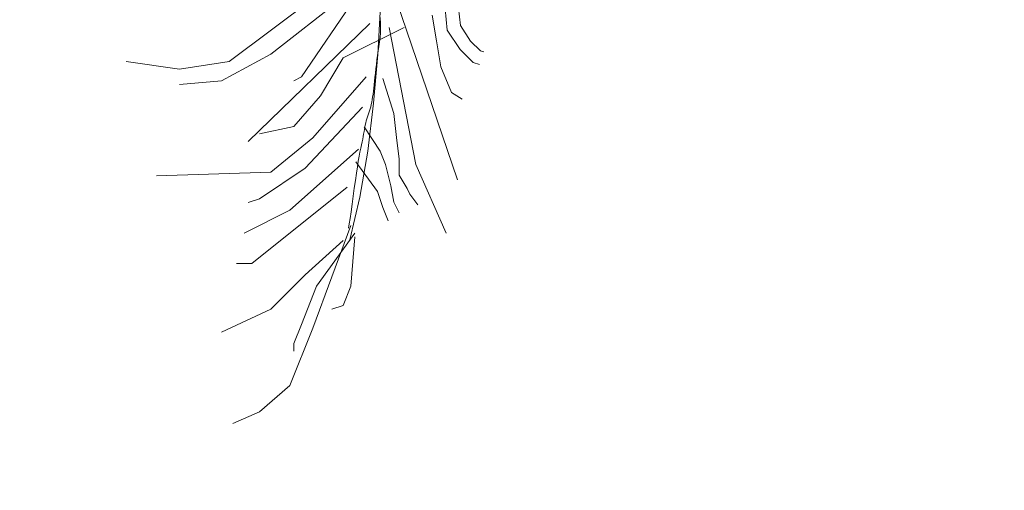
# Model space of a CAD drawing. Units: millimetres. Extents: x 595116 to 630915, y 909473 to 920225.
# Tile 83 of 134: x 629720.161 to 629727.558, y 919266.512 to 919270.048. Entities that reach past the tile are written whole.
import ezdxf

# ---------------------------------------------------------------- set-up
doc = ezdxf.new("R2010")
doc.units = ezdxf.units.MM
doc.layers.add('Dimension', color=3, linetype='Continuous', lineweight=18)
doc.layers.add('L-PLNT', color=85, linetype='Continuous', lineweight=13)
doc.styles.get("Standard").update_dxf_attribs({"font": 'arial.ttf'})
doc.dimstyles.new('ISO-25', dxfattribs={"dimtxt": 9, "dimasz": 6, "dimexe": 1.25, "dimexo": 0.625, "dimtad": 1, "dimlunit": 4, "dimtxsty": 'Standard', "dimcen": 2.5, "dimadec": 0, "dimazin": 0, "dimtfac": 1, "dimtmove": 0, "dimatfit": 3, "dimfxl": 1, "dimarcsym": 0})

# ---------------------------------------------------------------- blocks, each defined once
blk = doc.blocks.new('A$C4FB75ABC')
for p, q in [((3.325, 0.9299), (3.0505, 0.7241)), ((3.3098, 0.8766), (3.1344, 0.7394)), ((3.325, 0.8842), (3.1954, 0.6936)), ((3.3535, 0.836), (3.3484, 0.7387)), ((3.386, 0.8461), (3.508, 0.4878)), ((3.4831, 0.83), (3.4874, 0.787)), ((3.5101, 0.8314), (3.5136, 0.7963)), ((3.3521, 0.8161), (3.3535, 0.8034)), ((3.4573, 0.8171), (3.4659, 0.7655)), ((3.3326, 0.8003), (3.0886, 0.5641)), ((3.4013, 0.7927), (3.2793, 0.7317)), ((3.3535, 0.8034), (3.354, 0.7921)), ((3.354, 0.7921), (3.3537, 0.7819)), ((3.3708, 0.7927), (3.4242, 0.5183)), ((3.5136, 0.7963), (3.5342, 0.7654)), ((3.3529, 0.7725), (3.3517, 0.7635)), ((3.3537, 0.7819), (3.3529, 0.7725)), ((3.4874, 0.787), (3.5132, 0.7482)), ((3.3503, 0.7547), (3.349, 0.7457)), ((3.3517, 0.7635), (3.3503, 0.7547)), ((3.4659, 0.7655), (3.4745, 0.7138)), ((3.5342, 0.7654), (3.5536, 0.746)), ((3.1344, 0.7394), (3.0352, 0.686)), ((3.2793, 0.7317), (3.2335, 0.6555)), ((3.3484, 0.7387), (3.34, 0.641)), ((3.3478, 0.7367), (3.3466, 0.7276)), ((3.349, 0.7457), (3.3478, 0.7367)), ((3.5132, 0.7482), (3.5391, 0.7224)), ((3.5536, 0.746), (3.5605, 0.7437)), ((2.9513, 0.7089), (2.8446, 0.7241)), ((3.0505, 0.7241), (2.9513, 0.7089)), ((3.3445, 0.7097), (3.3435, 0.7011)), ((3.3455, 0.7186), (3.3445, 0.7097)), ((3.3466, 0.7276), (3.3455, 0.7186)), ((3.4745, 0.7138), (3.496, 0.6622)), ((3.5391, 0.7224), (3.552, 0.7181)), ((3.1954, 0.6936), (3.1801, 0.686)), ((3.325, 0.6936), (3.2182, 0.5717)), ((3.3426, 0.6929), (3.3417, 0.6851)), ((3.3435, 0.7011), (3.3426, 0.6929)), ((3.3586, 0.6905), (3.3801, 0.6206)), ((3.0352, 0.686), (2.9513, 0.6784)), ((3.3402, 0.6711), (3.3395, 0.6648)), ((3.341, 0.6779), (3.3402, 0.6711)), ((3.3417, 0.6851), (3.341, 0.6779)), ((3.2335, 0.6555), (3.1801, 0.5945)), ((3.338, 0.6533), (3.3372, 0.6481)), ((3.3388, 0.6589), (3.338, 0.6533)), ((3.3395, 0.6648), (3.3388, 0.6589)), ((3.496, 0.6622), (3.5175, 0.6493)), ((3.3174, 0.6327), (3.203, 0.5107)), ((3.34, 0.641), (3.3282, 0.5451)), ((3.3341, 0.634), (3.3329, 0.6297)), ((3.3353, 0.6385), (3.3341, 0.634)), ((3.3363, 0.6432), (3.3353, 0.6385)), ((3.3372, 0.6481), (3.3363, 0.6432)), ((3.3276, 0.6135), (3.3264, 0.6095)), ((3.3289, 0.6175), (3.3276, 0.6135)), ((3.3303, 0.6215), (3.3289, 0.6175)), ((3.3316, 0.6256), (3.3303, 0.6215)), ((3.3329, 0.6297), (3.3316, 0.6256)), ((3.3801, 0.6206), (3.3855, 0.5721)), ((3.1801, 0.5945), (3.1115, 0.5793)), ((3.3209, 0.5936), (3.3532, 0.5452)), ((3.3225, 0.593), (3.3216, 0.5886)), ((3.3233, 0.5973), (3.3225, 0.593)), ((3.3242, 0.6014), (3.3233, 0.5973)), ((3.3252, 0.6055), (3.3242, 0.6014)), ((3.3264, 0.6095), (3.3252, 0.6055)), ((3.2182, 0.5717), (3.1344, 0.5031)), ((3.3191, 0.5742), (3.3181, 0.5689)), ((3.32, 0.5792), (3.3191, 0.5742)), ((3.3208, 0.584), (3.32, 0.5792)), ((3.3216, 0.5886), (3.3208, 0.584)), ((3.3855, 0.5721), (3.3909, 0.5291)), ((3.3156, 0.5574), (3.3142, 0.5507)), ((3.3169, 0.5634), (3.3156, 0.5574)), ((3.3181, 0.5689), (3.3169, 0.5634)), ((3.3098, 0.5488), (3.1725, 0.4269)), ((3.3111, 0.5347), (3.3093, 0.5249)), ((3.3127, 0.5432), (3.3111, 0.5347)), ((3.3282, 0.5451), (3.3124, 0.4531)), ((3.3142, 0.5507), (3.3127, 0.5432)), ((3.3532, 0.5452), (3.364, 0.5183)), ((3.3047, 0.5237), (3.3478, 0.4645)), ((3.3075, 0.5137), (3.3055, 0.5008)), ((3.3093, 0.5249), (3.3075, 0.5137)), ((3.364, 0.5183), (3.3747, 0.4753)), ((3.3909, 0.5291), (3.3909, 0.4968)), ((3.4242, 0.5183), (3.4852, 0.3811)), ((3.1344, 0.5031), (2.9056, 0.4955)), ((3.203, 0.5107), (3.1115, 0.4497)), ((3.3055, 0.5008), (3.3034, 0.4863)), ((3.3909, 0.4968), (3.407, 0.4699)), ((3.3034, 0.4863), (3.3013, 0.4707)), ((3.3747, 0.4753), (3.3801, 0.443)), ((3.2869, 0.4726), (3.0962, 0.3201)), ((3.2992, 0.4546), (3.297, 0.4387)), ((3.3013, 0.4707), (3.2992, 0.4546)), ((3.3478, 0.4645), (3.3586, 0.4322)), ((3.407, 0.4699), (3.4124, 0.4591)), ((3.4124, 0.4591), (3.4286, 0.4376)), ((3.1115, 0.4497), (3.0886, 0.4421)), ((3.3124, 0.4531), (3.2923, 0.3674)), ((3.297, 0.4387), (3.2949, 0.4237)), ((3.3801, 0.443), (3.3909, 0.4214)), ((3.1725, 0.4269), (3.081, 0.3811)), ((3.2949, 0.4237), (3.2929, 0.4103)), ((3.3586, 0.4322), (3.3693, 0.4053)), ((3.2945, 0.3964), (3.2182, 0.1906)), ((3.2911, 0.3992), (3.2894, 0.3911)), ((3.2929, 0.4103), (3.2911, 0.3992)), ((3.3021, 0.3811), (3.2259, 0.2744)), ((3.2793, 0.3659), (3.203, 0.2973)), ((3.3021, 0.3735), (3.2945, 0.2744)), ((3.0962, 0.3201), (3.0657, 0.3201)), ((3.203, 0.2973), (3.1344, 0.2287)), ((3.2259, 0.2744), (3.1954, 0.1982)), ((3.2945, 0.2744), (3.2793, 0.2363)), ((3.1344, 0.2287), (3.0352, 0.1829)), ((3.2793, 0.2363), (3.2564, 0.2287)), ((3.1954, 0.1982), (3.1801, 0.1601)), ((3.2182, 0.1906), (3.1725, 0.0762)), ((3.1801, 0.1601), (3.1801, 0.1448)), ((3.1725, 0.0762), (3.1115, 0.0229)), ((3.1115, 0.0229), (3.0581, 0))]:
    blk.add_line(p, q)
blk = doc.blocks.new('*D216')
at = {"layer": 'Defpoints', "color": 0, "transparency": 16777216}
for p in [(629743.5408, 919411.9276), (629505.0408, 919411.8279), (629743.5408, 918832.3776)]:
    blk.add_point(p, dxfattribs=at)
at = {"layer": 'Dimension', "color": 0, "lineweight": -2, "transparency": 16777216}
for p, q in [((629743.5408, 919411.3026), (629743.5408, 918831.1276)), ((629505.0408, 919411.2029), (629505.0408, 918831.1276)), ((629511.0408, 918832.3776), (629737.5408, 918832.3776))]:
    blk.add_line(p, q, dxfattribs=at)
at = {"layer": 'Dimension', "color": 0, "transparency": 16777216}
for points in [[(629511.0408, 918833.3776), (629511.0408, 918831.3776), (629505.0408, 918832.3776)], [(629737.5408, 918833.3776), (629737.5408, 918831.3776), (629743.5408, 918832.3776)]]:
    blk.add_solid(points, dxfattribs=at)
at = {"layer": 'Dimension', "color": 0, "transparency": 16777216, "insert": (629624.2908, 918837.656), "char_height": 9, "attachment_point": 5}
blk.add_mtext('19\'-10 1/2"', dxfattribs=at)

msp = doc.modelspace()

# ---------------------------------------------------------------- block references
at = {"layer": 'L-PLNT', "xscale": 3.753413438031968, "yscale": 3.753413438031968, "zscale": 3.753413438031968}
msp.add_blockref('A$C4FB75ABC', (629710.2837, 919267.0144), dxfattribs=at)

# ---------------------------------------------------------------- dimensions: what is measured, and where the dimension line sits
at = {"layer": 'Dimension'}
dim = msp.add_linear_dim(base=(629743.5408, 918832.3776), p1=(629505.0408, 919411.8279), p2=(629743.5408, 919411.9276), dimstyle='ISO-25', override={"dimdec": 1, "dimlfac": 1, "dimrnd": 0, "dimzin": 1, "dimdsep": 46, "dimlunit": 4, "dimfrac": 2}, dxfattribs=at)
dim.commit()
dim.dimension.update_dxf_attribs({"geometry": '*D216', "text_midpoint": (629624.2908, 918837.656)})

doc.saveas('drawing.dxf')
